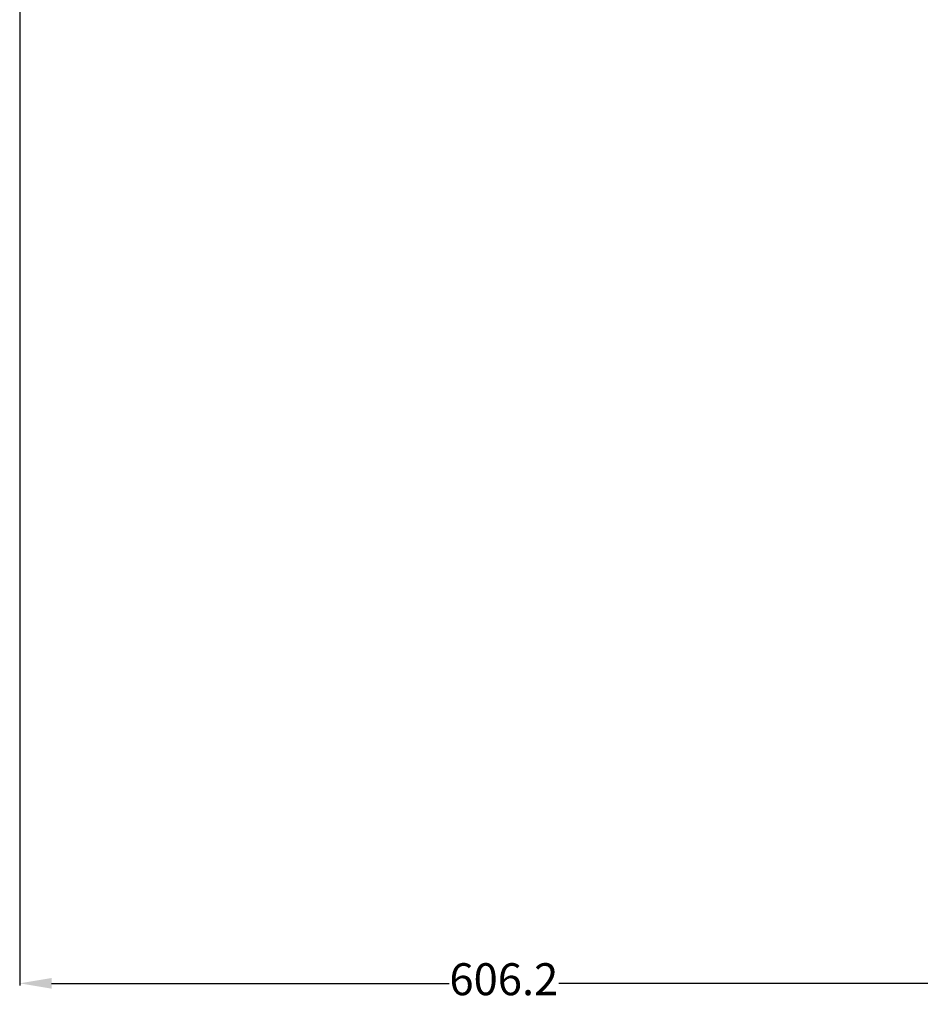
# Model space of a CAD drawing. Units: millimetres. Extents: x 78378 to 86415, y 148682 to 152721.
# Tile 6 of 18: x 80086 to 80650, y 148682 to 149298. Entities that reach past the tile are written whole.
import ezdxf

# ---------------------------------------------------------------- set-up
doc = ezdxf.new("R2010")
doc.units = ezdxf.units.MM
doc.layers.add('A-ANNO-DIMS', color=2, linetype='Continuous', lineweight=18)
doc.styles.get("Standard").update_dxf_attribs({"font": 'arial.ttf'})
doc.dimstyles.new('ISO-25', dxfattribs={"dimtxt": 20, "dimasz": 20, "dimexe": 1.25, "dimexo": 0.625, "dimtad": 0, "dimdec": 1, "dimtxsty": 'Standard', "dimcen": 2.5, "dimadec": 0, "dimazin": 0, "dimtfac": 1, "dimtdec": 1, "dimtmove": 0, "dimatfit": 3, "dimfxl": 1, "dimarcsym": 0})

# ---------------------------------------------------------------- blocks, each defined once
blk = doc.blocks.new('*D32')
at = {"layer": 'A-ANNO-DIMS', "color": 0, "lineweight": -2, "transparency": 16777216}
for p, q in [((80086.4, 150459.38), (80086.4, 148693.76)), ((80692.62, 150459.38), (80692.62, 148693.76)), ((80106.4, 148695.01), (80355.19, 148695.01)), ((80672.62, 148695.01), (80423.84, 148695.01))]:
    blk.add_line(p, q, dxfattribs=at)
at = {"layer": 'A-ANNO-DIMS', "color": 0, "transparency": 16777216}
for points in [[(80106.4, 148698.34), (80106.4, 148691.67), (80086.4, 148695.01)], [(80672.62, 148698.34), (80672.62, 148691.67), (80692.62, 148695.01)]]:
    blk.add_solid(points, dxfattribs=at)
at = {"layer": 'Defpoints', "color": 0, "transparency": 16777216}
for p in [(80086.4, 150460.01), (80692.62, 150460.01), (80692.62, 148695.01)]:
    blk.add_point(p, dxfattribs=at)
at = {"layer": 'A-ANNO-DIMS', "color": 0, "transparency": 16777216, "insert": (80389.51, 148695.01), "char_height": 20, "attachment_point": 5}
blk.add_mtext('606.2', dxfattribs=at)

msp = doc.modelspace()

# ---------------------------------------------------------------- dimensions: what is measured, and where the dimension line sits
at = {"layer": 'A-ANNO-DIMS'}
dim = msp.add_linear_dim(base=(80692.622, 148695.0076), p1=(80086.4042, 150460.0076), p2=(80692.622, 150460.0076), dimstyle='ISO-25', override={"dimdec": 1, "dimlfac": 1, "dimrnd": 0, "dimzin": 0, "dimdsep": 46, "dimlunit": 2}, dxfattribs=at)
dim.commit()
dim.dimension.update_dxf_attribs({"geometry": '*D32', "text_midpoint": (80389.5131, 148695.0076)})

doc.saveas('drawing.dxf')
